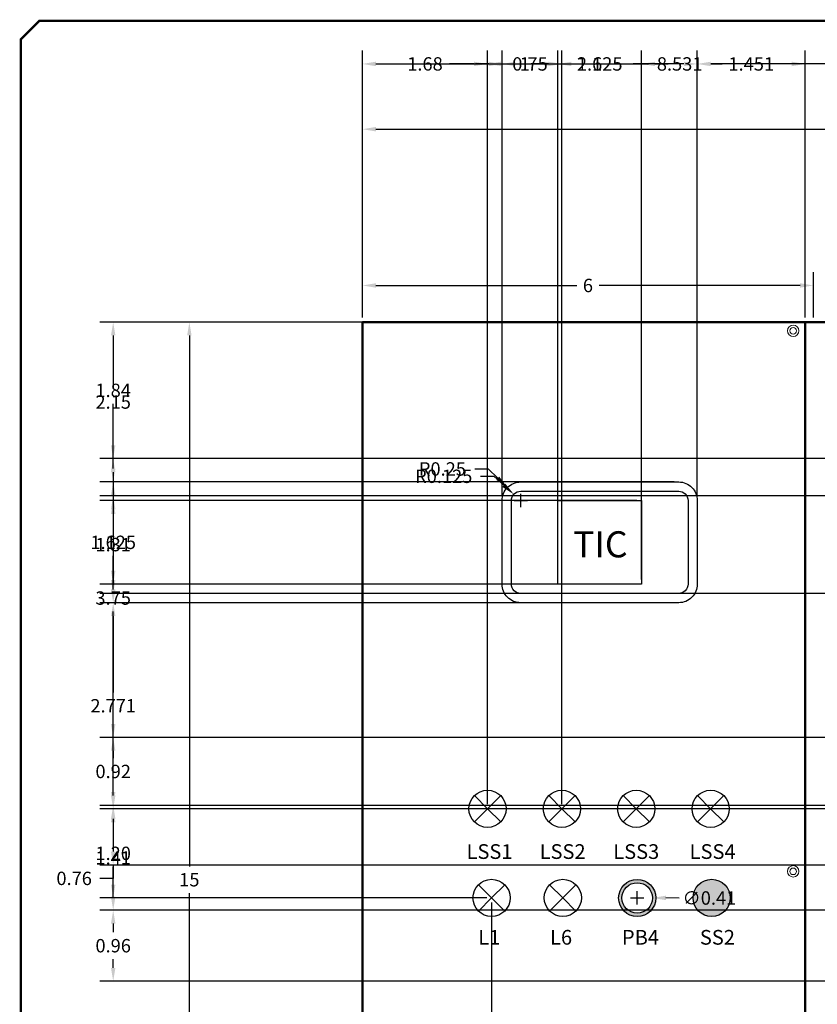
# Model space of a CAD drawing. Units: inches. Extents: x 0 to 33.5, y 0 to 22.4.
# Tile 2 of 6: x 0 to 10.7, y 9.2 to 22.4. Entities that reach past the tile are written whole.
import ezdxf
from ezdxf.enums import TextEntityAlignment as Align

# ---------------------------------------------------------------- set-up
doc = ezdxf.new("R2010")
doc.units = ezdxf.units.IN
doc.header["$MEASUREMENT"] = 0
for name, color, linetype, lineweight in [('E-ANNO-DIMS', 2, 'Continuous', 18), ('E-ANNO-TEXT', 7, 'Continuous', 18), ('E-ANNO-TTLB', 7, 'Continuous', 35), ('E-PANL-DEVC', 4, 'Continuous', 25), ('E-PANL-HDWR', 8, 'Continuous', 18), ('E-PANL-OUTL', 7, 'Continuous', 50), ('E-PANL-PATT', 8, 'Continuous', 13)]:
    doc.layers.add(name, color=color, linetype=linetype, lineweight=lineweight)
doc.layers.add('TITLE', color=7, linetype='Continuous')
doc.styles.add('ITALIC', font='ITALIC')
doc.styles.add('SIMPLEX', font='SIMPLEX')
doc.dimstyles.get("Standard").update_dxf_attribs({"dimtxt": 0.18, "dimasz": 0.18, "dimexe": 0.18, "dimexo": 0.0625, "dimgap": 0.09, "dimtad": 0, "dimtih": 1, "dimtoh": 1, "dimdec": 0, "dimzin": 0, "dimdsep": 46, "dimtxsty": 'Standard', "dimcen": 0.09, "dimadec": 0, "dimazin": 0, "dimtfac": 1, "dimtdec": 0, "dimtofl": 0, "dimtmove": 0, "dimatfit": 3, "dimfxl": 1, "dimtolj": 1, "dimtzin": 0, "dimarcsym": 0})

# ---------------------------------------------------------------- blocks, each defined once
blk = doc.blocks.new('NO_NUM_acade_title')
at = {"layer": 'TITLE', "const_width": 0.0312}
blk.add_lwpolyline([(30.594, 0.281), (30.594, 22.177), (30.344, 22.427), (0.281, 22.427), (0.031, 22.177), (0.031, 0.281), (0.281, 0.031), (30.344, 0.031)], close=True, dxfattribs=at)
at = {"layer": 'TITLE', "style": 'ITALIC'}
for tag, height, p in [('TITLE#1', 0.125, (32.156, 3.406)), ('TITLE#2', 0.125, (32.156, 3.204)), ('TITLE#3', 0.125, (32.156, 3.001)), ('TITLE#4', 0.125, (32.156, 2.799)), ('DWG#', 0.2, (32.156, 0.826))]:
    blk.add_attdef(tag, text='', height=height, dxfattribs=at).set_placement(p, align=Align.CENTER)
at = {"layer": 'TITLE', "style": 'SIMPLEX'}
blk.add_attdef('CAD#', (30.826, 1.958), '', height=0.0938, rotation=90, dxfattribs=at)
at = {"layer": 'TITLE'}
for tag, p, height, style in [('JOB#', (31.464, 1.644), 0.0938, 'SIMPLEX'), ('SCALE', (31.353, 1.344), 0.0938, 'SIMPLEX'), ('DATE', (32.408, 1.344), 0.0938, 'SIMPLEX'), ('SHTS', (32.532, 0.25), 0.2, 'ITALIC')]:
    blk.add_attdef(tag, p, '', height=height, dxfattribs=dict(at, style=style))
at = {"layer": 'TITLE', "style": 'ITALIC'}
blk.add_attdef('SH#', text='', height=0.2, dxfattribs=at).set_placement((31.881, 0.25), align=Align.RIGHT)
at = {"layer": 'TITLE', "flags": 9}
blk.add_attdef('WD_TB', (31.219, 0.031), '', height=0.125, dxfattribs=at)
blk = doc.blocks.new('*U9')
for q in [(-0.177, 0.177), (0.177, 0.177), (-0.177, -0.177), (0.177, -0.177)]:
    blk.add_line((0, 0), q)
blk.add_circle((0, 0), 0.25)
blk = doc.blocks.new('*U10')
at = {"layer": 'E-PANL-DEVC', "color": 0, "linetype": 'ByBlock', "lineweight": -2, "transparency": 16777216}
for p in [(0, 0), (1, 0), (2, 0), (3, 0)]:
    blk.add_blockref('*U9', p, dxfattribs=at)
blk = doc.blocks.new('*D17')
at = {"layer": 'Defpoints', "color": 0, "transparency": 16777216}
for p in [(4.625, 18.375), (2.297, 3.375), (4.625, 3.375)]:
    blk.add_point(p, dxfattribs=at)
at = {"layer": 'E-ANNO-DIMS', "color": 0, "lineweight": -2, "transparency": 16777216}
for p, q in [((4.563, 18.375), (2.117, 18.375)), ((2.297, 18.195), (2.297, 11.055)), ((2.297, 3.555), (2.297, 10.695)), ((4.563, 3.375), (2.117, 3.375))]:
    blk.add_line(p, q, dxfattribs=at)
at = {"layer": 'E-ANNO-DIMS', "color": 0, "transparency": 16777216}
for points in [[(2.267, 18.195), (2.327, 18.195), (2.297, 18.375)], [(2.267, 3.555), (2.327, 3.555), (2.297, 3.375)]]:
    blk.add_solid(points, dxfattribs=at)
at = {"layer": 'E-ANNO-DIMS', "color": 0, "transparency": 16777216, "insert": (2.297, 10.875), "char_height": 0.18, "attachment_point": 5}
blk.add_mtext('\\A1;15', dxfattribs=at)
blk = doc.blocks.new('*D18')
at = {"layer": 'Defpoints', "color": 0, "transparency": 16777216}
for p in [(23.794, 20.97), (4.625, 18.375), (23.794, 18.375)]:
    blk.add_point(p, dxfattribs=at)
at = {"layer": 'E-ANNO-DIMS', "color": 0, "lineweight": -2, "transparency": 16777216}
for p, q in [((4.625, 18.438), (4.625, 21.15)), ((23.794, 18.438), (23.794, 21.15)), ((4.805, 20.97), (13.999, 20.97)), ((23.614, 20.97), (14.419, 20.97))]:
    blk.add_line(p, q, dxfattribs=at)
at = {"layer": 'E-ANNO-DIMS', "color": 0, "transparency": 16777216}
for points in [[(4.805, 21), (4.805, 20.94), (4.625, 20.97)], [(23.614, 21), (23.614, 20.94), (23.794, 20.97)]]:
    blk.add_solid(points, dxfattribs=at)
at = {"layer": 'E-ANNO-DIMS', "color": 0, "transparency": 16777216, "insert": (14.209, 20.97), "char_height": 0.18, "attachment_point": 5}
blk.add_mtext('\\A1;19', dxfattribs=at)
blk = doc.blocks.new('*D19')
at = {"layer": 'Defpoints', "color": 0, "transparency": 16777216}
for p in [(4.625, 18.868), (4.625, 18.375), (10.689, 18.375)]:
    blk.add_point(p, dxfattribs=at)
at = {"layer": 'E-ANNO-DIMS', "color": 0, "lineweight": -2, "transparency": 16777216}
for p, q in [((4.625, 18.438), (4.625, 19.048)), ((10.689, 18.438), (10.689, 19.048)), ((4.805, 18.868), (7.507, 18.868)), ((10.509, 18.868), (7.807, 18.868))]:
    blk.add_line(p, q, dxfattribs=at)
at = {"layer": 'E-ANNO-DIMS', "color": 0, "transparency": 16777216}
for points in [[(4.805, 18.898), (4.805, 18.838), (4.625, 18.868)], [(10.509, 18.898), (10.509, 18.838), (10.689, 18.868)]]:
    blk.add_solid(points, dxfattribs=at)
at = {"layer": 'E-ANNO-DIMS', "color": 0, "transparency": 16777216, "insert": (7.657, 18.868), "char_height": 0.18, "attachment_point": 5}
blk.add_mtext('\\A1;6', dxfattribs=at)
blk = doc.blocks.new('LAMP-IND')
for q in [(0.073, 0.427), (0.426, 0.427), (0.073, 0.073), (0.426, 0.073)]:
    blk.add_line((0.25, 0.25), q)
blk.add_circle((0.25, 0.25), 0.25)
blk = doc.blocks.new('PB-FLUSH')
for radius in [0.25, 0.205]:
    blk.add_circle((0.25, 0.25), radius)
blk = doc.blocks.new('SCREW-PANEL')
for radius in [0.0768, 0.0442]:
    blk.add_circle((0.077, 0.077), radius)
blk = doc.blocks.new('*D30')
at = {"layer": 'Defpoints', "color": 0, "transparency": 16777216}
for p in [(13.156258, 21.847539), (4.625144, 18.375), (13.156258, 18.375)]:
    blk.add_point(p, dxfattribs=at)
at = {"layer": 'E-ANNO-DIMS', "color": 0, "lineweight": -2, "transparency": 16777216}
for p, q in [((4.625144, 18.4375), (4.625144, 22.027539)), ((13.156258, 18.4375), (13.156258, 22.027539)), ((4.805144, 21.847539), (8.470701, 21.847539)), ((12.976258, 21.847539), (9.310701, 21.847539))]:
    blk.add_line(p, q, dxfattribs=at)
at = {"layer": 'E-ANNO-DIMS', "color": 0, "transparency": 16777216}
for points in [[(4.805144, 21.877539), (4.805144, 21.817539), (4.625144, 21.847539)], [(12.976258, 21.877539), (12.976258, 21.817539), (13.156258, 21.847539)]]:
    blk.add_solid(points, dxfattribs=at)
at = {"layer": 'E-ANNO-DIMS', "color": 0, "transparency": 16777216, "insert": (8.890701, 21.847539), "char_height": 0.18, "attachment_point": 5}
blk.add_mtext('\\A1;8.531', dxfattribs=at)
blk = doc.blocks.new('*D39')
at = {"layer": 'Defpoints', "color": 0, "transparency": 16777216}
for p in [(9.127927, 21.847539), (6.502927, 15.975269), (9.127927, 15.975269)]:
    blk.add_point(p, dxfattribs=at)
at = {"layer": 'E-ANNO-DIMS', "color": 0, "lineweight": -2, "transparency": 16777216}
for p, q in [((6.502927, 16.037769), (6.502927, 22.027539)), ((9.127927, 16.037769), (9.127927, 22.027539)), ((6.682927, 21.847539), (7.365427, 21.847539)), ((8.947927, 21.847539), (8.265427, 21.847539))]:
    blk.add_line(p, q, dxfattribs=at)
at = {"layer": 'E-ANNO-DIMS', "color": 0, "transparency": 16777216}
for points in [[(6.682927, 21.877539), (6.682927, 21.817539), (6.502927, 21.847539)], [(8.947927, 21.877539), (8.947927, 21.817539), (9.127927, 21.847539)]]:
    blk.add_solid(points, dxfattribs=at)
at = {"layer": 'E-ANNO-DIMS', "color": 0, "transparency": 16777216, "insert": (7.815427, 21.847539), "char_height": 0.18, "attachment_point": 5}
blk.add_mtext('\\A1;2.625', dxfattribs=at)
blk = doc.blocks.new('*D40')
at = {"layer": 'Defpoints', "color": 0, "transparency": 16777216}
for p in [(8.877927, 16.225269), (1.272879, 14.600269), (8.877927, 14.600269)]:
    blk.add_point(p, dxfattribs=at)
at = {"layer": 'E-ANNO-DIMS', "color": 0, "lineweight": -2, "transparency": 16777216}
for p, q in [((8.815427, 16.225269), (1.092879, 16.225269)), ((1.272879, 16.045269), (1.272879, 15.592769)), ((1.272879, 14.780269), (1.272879, 15.232769)), ((8.815427, 14.600269), (1.092879, 14.600269))]:
    blk.add_line(p, q, dxfattribs=at)
at = {"layer": 'E-ANNO-DIMS', "color": 0, "transparency": 16777216}
for points in [[(1.242879, 16.045269), (1.302879, 16.045269), (1.272879, 16.225269)], [(1.242879, 14.780269), (1.302879, 14.780269), (1.272879, 14.600269)]]:
    blk.add_solid(points, dxfattribs=at)
at = {"layer": 'E-ANNO-DIMS', "color": 0, "transparency": 16777216, "insert": (1.272879, 15.412769), "char_height": 0.18, "attachment_point": 5}
blk.add_mtext('\\A1;1.625', dxfattribs=at)
blk = doc.blocks.new('*D41')
at = {"layer": 'Defpoints', "color": 0, "transparency": 16777216}
for p in [(8.377927, 21.847539), (7.252927, 14.850269), (8.377927, 14.850269)]:
    blk.add_point(p, dxfattribs=at)
at = {"layer": 'E-ANNO-DIMS', "color": 0, "lineweight": -2, "transparency": 16777216}
for p, q in [((7.252927, 14.912769), (7.252927, 22.027539)), ((8.377927, 14.912769), (8.377927, 22.027539)), ((7.072927, 21.847539), (6.892927, 21.847539)), ((8.557927, 21.847539), (8.737927, 21.847539))]:
    blk.add_line(p, q, dxfattribs=at)
at = {"layer": 'E-ANNO-DIMS', "color": 0, "transparency": 16777216}
for points in [[(7.072927, 21.877539), (7.072927, 21.817539), (7.252927, 21.847539)], [(8.557927, 21.877539), (8.557927, 21.817539), (8.377927, 21.847539)]]:
    blk.add_solid(points, dxfattribs=at)
at = {"layer": 'E-ANNO-DIMS', "color": 0, "transparency": 16777216, "insert": (7.815427, 21.847539), "char_height": 0.18, "attachment_point": 5}
blk.add_mtext('\\A1;1.125', dxfattribs=at)
blk = doc.blocks.new('*D42')
at = {"layer": 'Defpoints', "color": 0, "transparency": 16777216}
for p in [(8.377927, 15.975269), (1.272879, 14.850269), (8.377927, 14.850269)]:
    blk.add_point(p, dxfattribs=at)
at = {"layer": 'E-ANNO-DIMS', "color": 0, "lineweight": -2, "transparency": 16777216}
for p, q in [((8.315427, 15.975269), (1.092879, 15.975269)), ((1.272879, 15.795269), (1.272879, 15.592769)), ((1.272879, 15.030269), (1.272879, 15.232769)), ((8.315427, 14.850269), (1.092879, 14.850269))]:
    blk.add_line(p, q, dxfattribs=at)
at = {"layer": 'E-ANNO-DIMS', "color": 0, "transparency": 16777216}
for points in [[(1.242879, 15.795269), (1.302879, 15.795269), (1.272879, 15.975269)], [(1.242879, 15.030269), (1.302879, 15.030269), (1.272879, 14.850269)]]:
    blk.add_solid(points, dxfattribs=at)
at = {"layer": 'E-ANNO-DIMS', "color": 0, "transparency": 16777216, "insert": (1.272879, 15.412769), "char_height": 0.18, "attachment_point": 5}
blk.add_mtext('\\A1;1.125', dxfattribs=at)
blk = doc.blocks.new('*D43')
at = {"layer": 'Defpoints', "color": 0, "transparency": 16777216}
for p in [(7.252927, 21.847539), (6.502927, 15.975269), (7.252927, 15.975269)]:
    blk.add_point(p, dxfattribs=at)
at = {"layer": 'E-ANNO-DIMS', "color": 0, "lineweight": -2, "transparency": 16777216}
for p, q in [((6.502927, 16.037769), (6.502927, 22.027539)), ((7.252927, 16.037769), (7.252927, 22.027539)), ((6.322927, 21.847539), (6.142927, 21.847539)), ((7.432927, 21.847539), (7.612927, 21.847539))]:
    blk.add_line(p, q, dxfattribs=at)
at = {"layer": 'E-ANNO-DIMS', "color": 0, "transparency": 16777216}
for points in [[(6.322927, 21.877539), (6.322927, 21.817539), (6.502927, 21.847539)], [(7.432927, 21.877539), (7.432927, 21.817539), (7.252927, 21.847539)]]:
    blk.add_solid(points, dxfattribs=at)
at = {"layer": 'E-ANNO-DIMS', "color": 0, "transparency": 16777216, "insert": (6.877927, 21.847539), "char_height": 0.18, "attachment_point": 5}
blk.add_mtext('\\A1;0.75', dxfattribs=at)
blk = doc.blocks.new('*D44')
at = {"layer": 'Defpoints', "color": 0, "transparency": 16777216}
for p in [(10.578935, 21.847539), (10.578935, 18.375), (9.127927, 15.975269)]:
    blk.add_point(p, dxfattribs=at)
at = {"layer": 'E-ANNO-DIMS', "color": 0, "lineweight": -2, "transparency": 16777216}
for p, q in [((9.127927, 16.037769), (9.127927, 22.027539)), ((10.578935, 18.4375), (10.578935, 22.027539)), ((9.307927, 21.847539), (9.463431, 21.847539)), ((10.398935, 21.847539), (10.243431, 21.847539))]:
    blk.add_line(p, q, dxfattribs=at)
at = {"layer": 'E-ANNO-DIMS', "color": 0, "transparency": 16777216}
for points in [[(9.307927, 21.877539), (9.307927, 21.817539), (9.127927, 21.847539)], [(10.398935, 21.877539), (10.398935, 21.817539), (10.578935, 21.847539)]]:
    blk.add_solid(points, dxfattribs=at)
at = {"layer": 'E-ANNO-DIMS', "color": 0, "transparency": 16777216, "insert": (9.853431, 21.847539), "char_height": 0.18, "attachment_point": 5}
blk.add_mtext('\\A1;1.451', dxfattribs=at)
blk = doc.blocks.new('*D45')
at = {"layer": 'Defpoints', "color": 0, "transparency": 16777216}
for p in [(6.307, 21.848), (4.625, 18.375), (6.307, 11.829)]:
    blk.add_point(p, dxfattribs=at)
at = {"layer": 'E-ANNO-DIMS', "color": 0, "lineweight": -2, "transparency": 16777216}
for p, q in [((4.625, 18.438), (4.625, 22.028)), ((6.307, 11.892), (6.307, 22.028)), ((4.805, 21.848), (5.136, 21.848)), ((6.127, 21.848), (5.796, 21.848))]:
    blk.add_line(p, q, dxfattribs=at)
at = {"layer": 'E-ANNO-DIMS', "color": 0, "transparency": 16777216}
for points in [[(4.805, 21.878), (4.805, 21.818), (4.625, 21.848)], [(6.127, 21.878), (6.127, 21.818), (6.307, 21.848)]]:
    blk.add_solid(points, dxfattribs=at)
at = {"layer": 'E-ANNO-DIMS', "color": 0, "transparency": 16777216, "insert": (5.466, 21.848), "char_height": 0.18, "attachment_point": 5}
blk.add_mtext('\\A1;1.68', dxfattribs=at)
blk = doc.blocks.new('*D46')
at = {"layer": 'Defpoints', "color": 0, "transparency": 16777216}
for p in [(4.625, 18.375), (6.361, 10.63), (6.361, 0.355)]:
    blk.add_point(p, dxfattribs=at)
at = {"layer": 'E-ANNO-DIMS', "color": 0, "lineweight": -2, "transparency": 16777216}
for p, q in [((4.625, 18.312), (4.625, 0.175)), ((6.361, 10.568), (6.361, 0.175)), ((4.805, 0.355), (5.073, 0.355)), ((6.181, 0.355), (5.913, 0.355))]:
    blk.add_line(p, q, dxfattribs=at)
at = {"layer": 'E-ANNO-DIMS', "color": 0, "transparency": 16777216}
for points in [[(4.805, 0.385), (4.805, 0.325), (4.625, 0.355)], [(6.181, 0.385), (6.181, 0.325), (6.361, 0.355)]]:
    blk.add_solid(points, dxfattribs=at)
at = {"layer": 'E-ANNO-DIMS', "color": 0, "transparency": 16777216, "insert": (5.493, 0.355), "char_height": 0.18, "attachment_point": 5}
blk.add_mtext('\\A1;1.736', dxfattribs=at)
blk = doc.blocks.new('*D47')
at = {"layer": 'Defpoints', "color": 0, "transparency": 16777216}
for p in [(7.306787, 21.847539), (6.306787, 11.829032), (7.306787, 11.829032)]:
    blk.add_point(p, dxfattribs=at)
at = {"layer": 'E-ANNO-DIMS', "color": 0, "lineweight": -2, "transparency": 16777216}
for p, q in [((6.306787, 11.891532), (6.306787, 22.027539)), ((7.306787, 11.891532), (7.306787, 22.027539)), ((6.486787, 21.847539), (6.686787, 21.847539)), ((7.126787, 21.847539), (6.926787, 21.847539))]:
    blk.add_line(p, q, dxfattribs=at)
at = {"layer": 'E-ANNO-DIMS', "color": 0, "transparency": 16777216}
for points in [[(6.486787, 21.877539), (6.486787, 21.817539), (6.306787, 21.847539)], [(7.126787, 21.877539), (7.126787, 21.817539), (7.306787, 21.847539)]]:
    blk.add_solid(points, dxfattribs=at)
at = {"layer": 'E-ANNO-DIMS', "color": 0, "transparency": 16777216, "insert": (6.806787, 21.847539), "char_height": 0.18, "attachment_point": 5}
blk.add_mtext('\\A1;1', dxfattribs=at)
blk = doc.blocks.new('*D48')
at = {"layer": 'Defpoints', "color": 0, "transparency": 16777216}
for p in [(4.625, 18.375), (1.273, 16.225), (6.753, 16.225)]:
    blk.add_point(p, dxfattribs=at)
at = {"layer": 'E-ANNO-DIMS', "color": 0, "lineweight": -2, "transparency": 16777216}
for p, q in [((4.563, 18.375), (1.093, 18.375)), ((1.273, 18.195), (1.273, 17.48)), ((1.273, 16.405), (1.273, 17.12)), ((6.69, 16.225), (1.093, 16.225))]:
    blk.add_line(p, q, dxfattribs=at)
at = {"layer": 'E-ANNO-DIMS', "color": 0, "transparency": 16777216}
for points in [[(1.243, 18.195), (1.303, 18.195), (1.273, 18.375)], [(1.243, 16.405), (1.303, 16.405), (1.273, 16.225)]]:
    blk.add_solid(points, dxfattribs=at)
at = {"layer": 'E-ANNO-DIMS', "color": 0, "transparency": 16777216, "insert": (1.273, 17.3), "char_height": 0.18, "attachment_point": 5}
blk.add_mtext('\\A1;2.15', dxfattribs=at)
blk = doc.blocks.new('*D49')
at = {"layer": 'Defpoints', "color": 0, "transparency": 16777216}
for p in [(6.753, 14.6), (1.273, 11.829), (6.307, 11.829)]:
    blk.add_point(p, dxfattribs=at)
at = {"layer": 'E-ANNO-DIMS', "color": 0, "lineweight": -2, "transparency": 16777216}
for p, q in [((6.69, 14.6), (1.093, 14.6)), ((1.273, 14.42), (1.273, 13.395)), ((1.273, 12.009), (1.273, 13.035)), ((6.244, 11.829), (1.093, 11.829))]:
    blk.add_line(p, q, dxfattribs=at)
at = {"layer": 'E-ANNO-DIMS', "color": 0, "transparency": 16777216}
for points in [[(1.243, 14.42), (1.303, 14.42), (1.273, 14.6)], [(1.243, 12.009), (1.303, 12.009), (1.273, 11.829)]]:
    blk.add_solid(points, dxfattribs=at)
at = {"layer": 'E-ANNO-DIMS', "color": 0, "transparency": 16777216, "insert": (1.273, 13.215), "char_height": 0.18, "attachment_point": 5}
blk.add_mtext('\\A1;2.771', dxfattribs=at)
blk = doc.blocks.new('*D50')
at = {"layer": 'Defpoints', "color": 0, "transparency": 16777216}
for p in [(6.306787, 11.829032), (1.272879, 10.630354), (6.361261, 10.630354)]:
    blk.add_point(p, dxfattribs=at)
at = {"layer": 'E-ANNO-DIMS', "color": 0, "lineweight": -2, "transparency": 16777216}
for p, q in [((6.244287, 11.829032), (1.092879, 11.829032)), ((1.272879, 11.649032), (1.272879, 11.409693)), ((1.272879, 10.810354), (1.272879, 11.049693)), ((6.298761, 10.630354), (1.092879, 10.630354))]:
    blk.add_line(p, q, dxfattribs=at)
at = {"layer": 'E-ANNO-DIMS', "color": 0, "transparency": 16777216}
for points in [[(1.242879, 11.649032), (1.302879, 11.649032), (1.272879, 11.829032)], [(1.242879, 10.810354), (1.302879, 10.810354), (1.272879, 10.630354)]]:
    blk.add_solid(points, dxfattribs=at)
at = {"layer": 'E-ANNO-DIMS', "color": 0, "transparency": 16777216, "insert": (1.272879, 11.229693), "char_height": 0.18, "attachment_point": 5}
blk.add_mtext('\\A1;1.20', dxfattribs=at)
blk = doc.blocks.new('*D54')
at = {"layer": 'Defpoints', "color": 0, "transparency": 16777216}
for p in [(14.061773, 16.038508), (1.272879, 14.726008), (14.061773, 14.726008)]:
    blk.add_point(p, dxfattribs=at)
at = {"layer": 'E-ANNO-DIMS', "color": 0, "lineweight": -2, "transparency": 16777216}
for p, q in [((13.999273, 16.038508), (1.092879, 16.038508)), ((1.272879, 15.858508), (1.272879, 15.562258)), ((1.272879, 14.906008), (1.272879, 15.202258)), ((13.999273, 14.726008), (1.092879, 14.726008))]:
    blk.add_line(p, q, dxfattribs=at)
at = {"layer": 'E-ANNO-DIMS', "color": 0, "transparency": 16777216}
for points in [[(1.242879, 15.858508), (1.302879, 15.858508), (1.272879, 16.038508)], [(1.242879, 14.906008), (1.302879, 14.906008), (1.272879, 14.726008)]]:
    blk.add_solid(points, dxfattribs=at)
at = {"layer": 'E-ANNO-DIMS', "color": 0, "transparency": 16777216, "insert": (1.272879, 15.382258), "char_height": 0.18, "attachment_point": 5}
blk.add_mtext('\\A1;1.31', dxfattribs=at)
blk = doc.blocks.new('*D59')
at = {"layer": 'Defpoints', "color": 0, "transparency": 16777216}
for p in [(10.793806, 18.375), (1.272879, 16.538508), (12.811773, 16.538508)]:
    blk.add_point(p, dxfattribs=at)
at = {"layer": 'E-ANNO-DIMS', "color": 0, "lineweight": -2, "transparency": 16777216}
for p, q in [((10.731306, 18.375), (1.092879, 18.375)), ((1.272879, 18.195), (1.272879, 17.636754)), ((1.272879, 16.718508), (1.272879, 17.276754)), ((12.749273, 16.538508), (1.092879, 16.538508))]:
    blk.add_line(p, q, dxfattribs=at)
at = {"layer": 'E-ANNO-DIMS', "color": 0, "transparency": 16777216}
for points in [[(1.242879, 18.195), (1.302879, 18.195), (1.272879, 18.375)], [(1.242879, 16.718508), (1.302879, 16.718508), (1.272879, 16.538508)]]:
    blk.add_solid(points, dxfattribs=at)
at = {"layer": 'E-ANNO-DIMS', "color": 0, "transparency": 16777216, "insert": (1.272879, 17.456754), "char_height": 0.18, "attachment_point": 5}
blk.add_mtext('\\A1;1.84', dxfattribs=at)
blk = doc.blocks.new('*D60')
at = {"layer": 'Defpoints', "color": 0, "transparency": 16777216}
for p in [(12.811773, 16.538508), (1.272879, 12.788508), (12.811773, 12.788508)]:
    blk.add_point(p, dxfattribs=at)
at = {"layer": 'E-ANNO-DIMS', "color": 0, "lineweight": -2, "transparency": 16777216}
for p, q in [((12.749273, 16.538508), (1.092879, 16.538508)), ((1.272879, 16.358508), (1.272879, 14.843508)), ((1.272879, 12.968508), (1.272879, 14.483508)), ((12.749273, 12.788508), (1.092879, 12.788508))]:
    blk.add_line(p, q, dxfattribs=at)
at = {"layer": 'E-ANNO-DIMS', "color": 0, "transparency": 16777216}
for points in [[(1.242879, 16.358508), (1.302879, 16.358508), (1.272879, 16.538508)], [(1.242879, 12.968508), (1.302879, 12.968508), (1.272879, 12.788508)]]:
    blk.add_solid(points, dxfattribs=at)
at = {"layer": 'E-ANNO-DIMS', "color": 0, "transparency": 16777216, "insert": (1.272879, 14.663508), "char_height": 0.18, "attachment_point": 5}
blk.add_mtext('\\A1;3.75', dxfattribs=at)
blk = doc.blocks.new('*D61')
at = {"layer": 'Defpoints', "color": 0, "transparency": 16777216}
for p in [(12.812, 12.789), (1.273, 11.873), (12.996, 11.873)]:
    blk.add_point(p, dxfattribs=at)
at = {"layer": 'E-ANNO-DIMS', "color": 0, "lineweight": -2, "transparency": 16777216}
for p, q in [((12.749, 12.789), (1.093, 12.789)), ((1.273, 12.609), (1.273, 12.511)), ((1.273, 12.053), (1.273, 12.151)), ((12.933, 11.873), (1.093, 11.873))]:
    blk.add_line(p, q, dxfattribs=at)
at = {"layer": 'E-ANNO-DIMS', "color": 0, "transparency": 16777216}
for points in [[(1.243, 12.609), (1.303, 12.609), (1.273, 12.789)], [(1.243, 12.053), (1.303, 12.053), (1.273, 11.873)]]:
    blk.add_solid(points, dxfattribs=at)
at = {"layer": 'E-ANNO-DIMS', "color": 0, "transparency": 16777216, "insert": (1.273, 12.331), "char_height": 0.18, "attachment_point": 5}
blk.add_mtext('\\A1;0.92', dxfattribs=at)
blk = doc.blocks.new('*D62')
at = {"layer": 'Defpoints', "color": 0, "transparency": 16777216}
for p in [(12.996, 11.873), (1.273, 10.465), (12.996, 10.465)]:
    blk.add_point(p, dxfattribs=at)
at = {"layer": 'E-ANNO-DIMS', "color": 0, "lineweight": -2, "transparency": 16777216}
for p, q in [((12.933, 11.873), (1.093, 11.873)), ((1.273, 11.693), (1.273, 11.349)), ((1.273, 10.645), (1.273, 10.989)), ((12.933, 10.465), (1.093, 10.465))]:
    blk.add_line(p, q, dxfattribs=at)
at = {"layer": 'E-ANNO-DIMS', "color": 0, "transparency": 16777216}
for points in [[(1.243, 11.693), (1.303, 11.693), (1.273, 11.873)], [(1.243, 10.645), (1.303, 10.645), (1.273, 10.465)]]:
    blk.add_solid(points, dxfattribs=at)
at = {"layer": 'E-ANNO-DIMS', "color": 0, "transparency": 16777216, "insert": (1.273, 11.169), "char_height": 0.18, "attachment_point": 5}
blk.add_mtext('\\A1;1.41', dxfattribs=at)
blk = doc.blocks.new('*D63')
at = {"layer": 'Defpoints', "color": 0, "transparency": 16777216}
for p in [(12.995825, 10.465374), (1.272879, 9.509708), (13.047227, 9.509708)]:
    blk.add_point(p, dxfattribs=at)
at = {"layer": 'E-ANNO-DIMS', "color": 0, "lineweight": -2, "transparency": 16777216}
for p, q in [((12.933325, 10.465374), (1.092879, 10.465374)), ((1.272879, 10.285374), (1.272879, 10.167541)), ((1.272879, 9.689708), (1.272879, 9.807541)), ((12.984727, 9.509708), (1.092879, 9.509708))]:
    blk.add_line(p, q, dxfattribs=at)
at = {"layer": 'E-ANNO-DIMS', "color": 0, "transparency": 16777216}
for points in [[(1.242879, 10.285374), (1.302879, 10.285374), (1.272879, 10.465374)], [(1.242879, 9.689708), (1.302879, 9.689708), (1.272879, 9.509708)]]:
    blk.add_solid(points, dxfattribs=at)
at = {"layer": 'E-ANNO-DIMS', "color": 0, "transparency": 16777216, "insert": (1.272879, 9.987541), "char_height": 0.18, "attachment_point": 5}
blk.add_mtext('\\A1;0.96', dxfattribs=at)
blk = doc.blocks.new('*D86')
at = {"layer": 'Defpoints', "color": 0, "transparency": 16777216}
for p in [(19.972101, 11.828212), (1.272879, 11.072826), (19.972101, 11.072826)]:
    blk.add_point(p, dxfattribs=at)
at = {"layer": 'E-ANNO-DIMS', "color": 0, "lineweight": -2, "transparency": 16777216}
for p, q in [((19.909601, 11.828212), (1.092879, 11.828212)), ((1.272879, 11.648212), (1.272879, 11.252826)), ((19.909601, 11.072826), (1.092879, 11.072826)), ((1.272879, 11.072826), (1.272879, 10.892826)), ((1.272879, 10.892826), (1.092879, 10.892826))]:
    blk.add_line(p, q, dxfattribs=at)
at = {"layer": 'E-ANNO-DIMS', "color": 0, "transparency": 16777216}
for points in [[(1.242879, 11.648212), (1.302879, 11.648212), (1.272879, 11.828212)], [(1.242879, 11.252826), (1.302879, 11.252826), (1.272879, 11.072826)]]:
    blk.add_solid(points, dxfattribs=at)
at = {"layer": 'E-ANNO-DIMS', "color": 0, "transparency": 16777216, "insert": (0.747879, 10.892826), "char_height": 0.18, "attachment_point": 5}
blk.add_mtext('\\A1;0.76', dxfattribs=at)
blk = doc.blocks.new('*D88')
at = {"layer": 'Defpoints', "color": 0, "transparency": 16777216}
for p in [(6.574, 16.149), (6.753, 15.975)]:
    blk.add_point(p, dxfattribs=at)
at = {"layer": 'E-ANNO-DIMS', "color": 0, "lineweight": -2, "transparency": 16777216}
for p, q in [((6.135, 16.4), (6.315, 16.4)), ((6.315, 16.4), (6.444, 16.275)), ((6.753, 15.885), (6.753, 16.065)), ((6.663, 15.975), (6.843, 15.975))]:
    blk.add_line(p, q, dxfattribs=at)
at = {"layer": 'E-ANNO-DIMS', "color": 0, "transparency": 16777216}
blk.add_solid([(6.465, 16.296), (6.423, 16.253), (6.574, 16.149)], dxfattribs=at)
at = {"layer": 'E-ANNO-DIMS', "color": 0, "transparency": 16777216, "insert": (5.7, 16.4), "char_height": 0.18, "attachment_point": 5}
blk.add_mtext('\\A1;R0.25', dxfattribs=at)
blk = doc.blocks.new('*D89')
at = {"layer": 'Defpoints', "color": 0, "transparency": 16777216}
for p in [(6.66, 16.059), (6.753, 15.975)]:
    blk.add_point(p, dxfattribs=at)
at = {"layer": 'E-ANNO-DIMS', "color": 0, "lineweight": -2, "transparency": 16777216}
for p, q in [((6.213, 16.301), (6.393, 16.301)), ((6.393, 16.301), (6.527, 16.18)), ((6.753, 15.885), (6.753, 16.065)), ((6.663, 15.975), (6.843, 15.975))]:
    blk.add_line(p, q, dxfattribs=at)
at = {"layer": 'E-ANNO-DIMS', "color": 0, "transparency": 16777216}
blk.add_solid([(6.547, 16.202), (6.507, 16.158), (6.66, 16.059)], dxfattribs=at)
at = {"layer": 'E-ANNO-DIMS', "color": 0, "transparency": 16777216, "insert": (5.718, 16.301), "char_height": 0.18, "attachment_point": 5}
blk.add_mtext('\\A1;R0.125', dxfattribs=at)
blk = doc.blocks.new('*D90')
at = {"layer": 'Defpoints', "color": 0, "transparency": 16777216}
for p in [(8.115, 10.631), (8.525, 10.63)]:
    blk.add_point(p, dxfattribs=at)
at = {"layer": 'E-ANNO-DIMS', "color": 0, "lineweight": -2, "transparency": 16777216}
for p, q in [((8.23, 10.63), (8.41, 10.63)), ((8.32, 10.54), (8.32, 10.72)), ((8.885, 10.629), (8.705, 10.63))]:
    blk.add_line(p, q, dxfattribs=at)
at = {"layer": 'E-ANNO-DIMS', "color": 0, "transparency": 16777216}
blk.add_solid([(8.705, 10.66), (8.705, 10.6), (8.525, 10.63)], dxfattribs=at)
at = {"layer": 'E-ANNO-DIMS', "color": 0, "transparency": 16777216, "insert": (9.29, 10.629), "char_height": 0.18, "attachment_point": 5}
blk.add_mtext('\\A1;∅0.41', dxfattribs=at)

msp = doc.modelspace()

# ---------------------------------------------------------------- hatches: boundary and pattern name
at = {"layer": 'E-PANL-PATT'}
h = msp.add_hatch(color=256, dxfattribs=at)
h.dxf.hatch_style = 1
h.paths.add_polyline_path([(9.0712, 10.6304, 1), (9.5712, 10.6304, 1)])
h.paths.add_polyline_path([(8.5702, 10.6304, 1), (8.0702, 10.6304, 1)])
h.paths.add_polyline_path([(8.115, 10.6304, -1), (8.5254, 10.6304, -1)], flags=16)
h.paths.add_polyline_path([(13.2972, 9.5097, 1), (12.7972, 9.5097, 1)])
h.paths.add_polyline_path([(12.842, 9.5097, -1), (13.2524, 9.5097, -1)], flags=16)

# ---------------------------------------------------------------- linework, layer by layer
at = {"layer": 'E-PANL-DEVC'}
for points in [[(6.5029, 15.9753, -0.4142136), (6.7529, 16.2253), (8.8779, 16.2253, -0.4142136), (9.1279, 15.9753), (9.1279, 14.8503, -0.4142136), (8.8779, 14.6003), (6.7529, 14.6003, -0.4142136), (6.5029, 14.8503)], [(6.6279, 15.9753, -0.4142136), (6.7529, 16.1003), (8.8779, 16.1003, -0.4142136), (9.0029, 15.9753), (9.0029, 14.8503, -0.4142136), (8.8779, 14.7253), (6.7529, 14.7253, -0.4142136), (6.6279, 14.8503)]]:
    msp.add_lwpolyline(points, format="xyb", close=True, dxfattribs=at)
msp.add_lwpolyline([(7.2529, 15.9753), (8.3779, 15.9753), (8.3779, 14.8503), (7.2529, 14.8503)], close=True, dxfattribs=at)
msp.add_circle((9.3212, 10.6304), 0.25, dxfattribs=at)
at = {"layer": 'E-PANL-OUTL'}
for p, q in [((4.6251, 18.375), (23.7937, 18.375)), ((4.6251, 3.375), (4.6251, 18.375)), ((10.5789, 3.5899), (10.5789, 18.375))]:
    msp.add_line(p, q, dxfattribs=at)

# ---------------------------------------------------------------- block references
at = {"layer": 'E-ANNO-TTLB'}
msp.add_blockref('NO_NUM_acade_title', (0, 0), dxfattribs=at)
at = {"layer": 'E-PANL-DEVC'}
for name, p in [('*U10', (6.3068, 11.829)), ('PB-FLUSH', (8.07, 10.38))]:
    msp.add_blockref(name, p, dxfattribs=at)
for p, rotation in [((6.6112, 10.3807), 90.0000000000013), ((7.5691, 10.3807), 90.00000000000146)]:
    msp.add_blockref('LAMP-IND', p, dxfattribs=dict(at, rotation=rotation))
at = {"layer": 'E-PANL-HDWR'}
for p in [(10.341, 18.182), (10.341, 10.9105)]:
    msp.add_blockref('SCREW-PANEL', p, dxfattribs=at)

# ---------------------------------------------------------------- texts
at = {"layer": 'E-ANNO-TEXT'}
for s, height, p in [('TIC', 0.35114, (7.4577, 15.2105)), ('LSS1', 0.19791, (6.0247, 11.1547)), ('LSS2', 0.19791, (7.0075, 11.1547)), ('LSS3', 0.19791, (7.9977, 11.1547)), ('LSS4', 0.19791, (9.0245, 11.1547)), ('L1', 0.19791, (6.1812, 10.0015)), ('L6', 0.19791, (7.1477, 10.0015)), ('PB4', 0.19791, (8.1142, 10.0015)), ('SS2', 0.19791, (9.1622, 10.0015))]:
    msp.add_text(s, height=height, dxfattribs=at).set_placement(p)

# ---------------------------------------------------------------- dimensions: what is measured, and where the dimension line sits
at = {"layer": 'E-ANNO-DIMS'}
for base, p1, p2, override, picture, middle in [((13.1563, 21.8475), (4.6251, 18.375), (13.1563, 18.375), {"dimdec": 3, "dimlfac": 1, "dimrnd": 0, "dimzin": 0, "dimdsep": 46, "dimlunit": 2}, '*D30', (8.8907, 21.8475)), ((6.3068, 21.8475), (4.6251, 18.375), (6.3068, 11.829), {"dimdec": 2, "dimlfac": 1, "dimrnd": 0, "dimzin": 0, "dimdsep": 46, "dimlunit": 2}, '*D45', (5.466, 21.8475)), ((7.2529, 21.8475), (6.5029, 15.9753), (7.2529, 15.9753), {"dimdec": 2, "dimlfac": 1, "dimrnd": 0, "dimzin": 0, "dimdsep": 46, "dimlunit": 2}, '*D43', (6.8779, 21.8475)), ((7.3068, 21.8475), (6.3068, 11.829), (7.3068, 11.829), {"dimdec": 0, "dimlfac": 1, "dimrnd": 0, "dimzin": 0, "dimdsep": 46, "dimlunit": 2}, '*D47', (6.8068, 21.8475)), ((9.1279, 21.8475), (6.5029, 15.9753), (9.1279, 15.9753), {"dimdec": 3, "dimlfac": 1, "dimrnd": 0, "dimzin": 0, "dimdsep": 46, "dimlunit": 2}, '*D39', (7.8154, 21.8475)), ((8.3779, 21.8475), (7.2529, 14.8503), (8.3779, 14.8503), {"dimdec": 3, "dimlfac": 1, "dimrnd": 0, "dimzin": 0, "dimdsep": 46, "dimlunit": 2}, '*D41', (7.8154, 21.8475)), ((10.5789, 21.8475), (9.1279, 15.9753), (10.5789, 18.375), {"dimdec": 3, "dimlfac": 1, "dimrnd": 0, "dimzin": 0, "dimdsep": 46, "dimlunit": 2}, '*D44', (9.8534, 21.8475)), ((23.7937, 20.9702), (4.6251, 18.375), (23.7937, 18.375), {"dimclrd": 0, "dimclre": 0, "dimclrt": 0}, '*D18', (14.2094, 20.9702)), ((4.6251, 18.8681), (10.6894, 18.375), (4.6251, 18.375), {"dimclrd": 0, "dimclre": 0, "dimclrt": 0}, '*D19', (7.6573, 18.8681)), ((6.3613, 0.3546), (4.6251, 18.375), (6.3613, 10.6304), {"dimdec": 3, "dimlfac": 1, "dimrnd": 0, "dimzin": 0, "dimdsep": 46, "dimlunit": 2}, '*D46', (5.4932, 0.3546))]:
    dim = msp.add_linear_dim(base=base, p1=p1, p2=p2, dimstyle='Standard', override=override, dxfattribs=at)
    dim.commit()
    dim.dimension.update_dxf_attribs({"geometry": picture, "text_midpoint": middle})
for base, p1, p2, override, picture, middle in [((1.2729, 16.2253), (4.6251, 18.375), (6.7529, 16.2253), {"dimdec": 2, "dimlfac": 1, "dimrnd": 0, "dimzin": 0, "dimdsep": 46, "dimlunit": 2}, '*D48', (1.2729, 17.3001)), ((1.2729, 16.5385), (10.7938, 18.375), (12.8118, 16.5385), {"dimdec": 2, "dimlfac": 1, "dimrnd": 0, "dimzin": 0, "dimdsep": 46, "dimlunit": 2}, '*D59', (1.2729, 17.4568)), ((2.2967, 3.375), (4.6251, 18.375), (4.6251, 3.375), {"dimclrd": 0, "dimclre": 0, "dimclrt": 0}, '*D17', (2.2967, 10.875)), ((1.2729, 12.7885), (12.8118, 16.5385), (12.8118, 12.7885), {"dimdec": 2, "dimlfac": 1, "dimrnd": 0, "dimzin": 0, "dimdsep": 46, "dimlunit": 2}, '*D60', (1.2729, 14.6635)), ((1.2729, 14.6003), (8.8779, 16.2253), (8.8779, 14.6003), {"dimdec": 3, "dimlfac": 1, "dimrnd": 0, "dimzin": 0, "dimdsep": 46, "dimlunit": 2}, '*D40', (1.2729, 15.4128)), ((1.2729, 14.726), (14.0618, 16.0385), (14.0618, 14.726), {"dimdec": 2, "dimlfac": 1, "dimrnd": 0, "dimzin": 0, "dimdsep": 46, "dimlunit": 2}, '*D54', (1.2729, 15.3823)), ((1.2729, 14.8503), (8.3779, 15.9753), (8.3779, 14.8503), {"dimdec": 3, "dimlfac": 1, "dimrnd": 0, "dimzin": 0, "dimdsep": 46, "dimlunit": 2}, '*D42', (1.2729, 15.4128)), ((1.2729, 11.829), (6.7529, 14.6003), (6.3068, 11.829), {"dimdec": 3, "dimlfac": 1, "dimrnd": 0, "dimzin": 0, "dimdsep": 46, "dimlunit": 2}, '*D49', (1.2729, 13.2147)), ((1.2729, 11.8727), (12.8118, 12.7885), (12.9958, 11.8727), {"dimdec": 2, "dimlfac": 1, "dimrnd": 0, "dimzin": 0, "dimdsep": 46, "dimlunit": 2}, '*D61', (1.2729, 12.3306)), ((1.2729, 11.0728), (19.9721, 11.8282), (19.9721, 11.0728), {"dimdec": 2, "dimlfac": 1, "dimrnd": 0, "dimzin": 0, "dimdsep": 46, "dimlunit": 2}, '*D86', (0.7479, 10.8928)), ((1.2729, 10.4654), (12.9958, 11.8727), (12.9958, 10.4654), {"dimdec": 2, "dimlfac": 1, "dimrnd": 0, "dimzin": 0, "dimdsep": 46, "dimlunit": 2}, '*D62', (1.2729, 11.169)), ((1.2729, 10.6304), (6.3068, 11.829), (6.3613, 10.6304), {"dimdec": 2, "dimlfac": 1, "dimrnd": 0, "dimzin": 0, "dimdsep": 46, "dimlunit": 2}, '*D50', (1.2729, 11.2297)), ((1.2729, 9.5097), (12.9958, 10.4654), (13.0472, 9.5097), {"dimdec": 2, "dimlfac": 1, "dimrnd": 0, "dimzin": 0, "dimdsep": 46, "dimlunit": 2}, '*D63', (1.2729, 9.9875))]:
    dim = msp.add_linear_dim(base=base, p1=p1, p2=p2, angle=90, dimstyle='Standard', override=override, dxfattribs=at)
    dim.commit()
    dim.dimension.update_dxf_attribs({"geometry": picture, "text_midpoint": middle})
for mpoint, override, picture, middle in [((6.5735, 16.1494), {"dimdec": 2, "dimlfac": 1, "dimrnd": 0, "dimzin": 0, "dimdsep": 46, "dimlunit": 2}, '*D88', (5.7001, 16.4001)), ((6.6602, 16.0591), {"dimdec": 3, "dimlfac": 1, "dimrnd": 0, "dimzin": 0, "dimdsep": 46, "dimlunit": 2}, '*D89', (5.7183, 16.3006))]:
    dim = msp.add_radius_dim(center=(6.7529, 15.9753), mpoint=mpoint, dimstyle='Standard', override=override, dxfattribs=at)
    dim.commit()
    dim.dimension.update_dxf_attribs({"geometry": picture, "text_midpoint": middle})
dim = msp.add_diameter_dim_2p(p1=(8.115, 10.6307), p2=(8.5254, 10.63), dimstyle='Standard', override={"dimdec": 2, "dimlfac": 1, "dimrnd": 0, "dimzin": 0, "dimdsep": 46, "dimlunit": 2}, dxfattribs=at)
dim.commit()
dim.dimension.update_dxf_attribs({"geometry": '*D90', "text_midpoint": (8.8854, 10.6294)})

doc.saveas('drawing.dxf')
